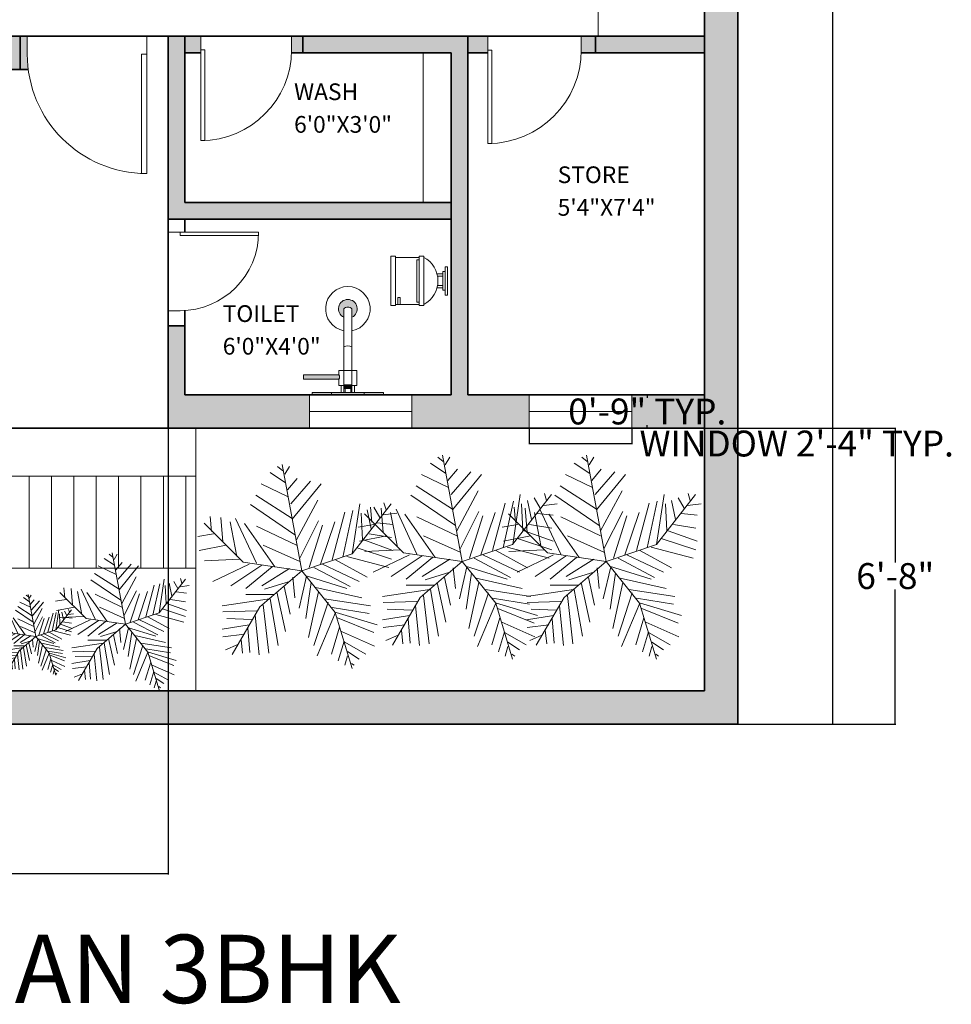
# Model space of a CAD drawing. Units: inches. Extents: x 1319 to 2030, y 219 to 1069.
# Tile 22 of 28: x 1776 to 2028, y 219 to 486. Entities that reach past the tile are written whole.
import ezdxf

# ---------------------------------------------------------------- set-up
doc = ezdxf.new("R2010")
doc.units = ezdxf.units.IN
doc.header["$MEASUREMENT"] = 0
doc.layers.get('0').update_dxf_attribs({"color": 12})
for name, color, linetype, lineweight in [('A-ANNO-DIMS', 2, 'Continuous', 18), ('A-AREA-IDEN', 250, 'Continuous', 18), ('A-FLOR', 8, 'Continuous', 18), ('A-FLOR-CASE', 8, 'Continuous', 18), ('A-FLOR-PATT', 41, 'Continuous', 13), ('A-GLAZ', 4, 'Continuous', 18), ('A-WALL-PATT', 252, 'Continuous', 13), ('C-PROP', 7, 'Continuous', 35), ('doors', 252, 'Continuous', 18), ('lawn', 82, 'Continuous', 13), ('PLUMBING FIXTURES', 252, 'Continuous', 18), ('text', 7, 'Continuous', 25), ('walls', 250, 'Continuous', 35)]:
    doc.layers.add(name, color=color, linetype=linetype, lineweight=lineweight)
doc.styles.get("Standard").update_dxf_attribs({"font": 'arial.ttf'})
doc.dimstyles.get("Standard").update_dxf_attribs({"dimtxt": 7, "dimasz": 0.18, "dimexe": 0.18, "dimexo": 0.0625, "dimgap": 0.09, "dimtad": 0, "dimtih": 1, "dimtoh": 1, "dimzin": 0, "dimdsep": 46, "dimlunit": 3, "dimtxsty": 'Standard', "dimcen": 0.09, "dimadec": 0, "dimazin": 0, "dimtfac": 1, "dimtofl": 0, "dimtmove": 0, "dimatfit": 3, "dimfxl": 1, "dimtolj": 1, "dimtzin": 0, "dimarcsym": 0})

# ---------------------------------------------------------------- blocks, each defined once
blk = doc.blocks.new('*U2')
for p, q in [((0, 0), (0, -6)), ((40, 0), (40, -6))]:
    blk.add_line(p, q)
blk.add_lwpolyline([(0, 0), (0, 40), (1.75, 40), (1.75, 0)], close=True)
blk.add_arc((0, 0), 40, 0, 90)
blk = doc.blocks.new('O.H SHOWER-PL')
at = {"layer": 'PLUMBING FIXTURES'}
for points in [[(-1.84, 0), (-1.84, -0.25), (1.84, -0.25), (1.84, 0)], [(0.46, -8.72), (0.46, -9.67, -0.422337), (-0.46, -9.67), (-0.46, -8.72, 4.325472)]]:
    blk.add_hatch(color=256, dxfattribs=at).paths.add_polyline_path(points)
for p, q in [((-1.84, 0), (-1.84, -0.25)), ((1.84, 0), (-1.84, 0)), ((1.84, 0), (1.84, -0.25)), ((1.84, -0.25), (-1.84, -0.25)), ((-0.46, -0.25), (-0.46, -9.67)), ((0.46, -0.25), (0.46, -9.67))]:
    blk.add_line(p, q, dxfattribs=at)
for centre, radius, start, end in [((0, -4.48), 1.03, 243.53, 296.47), ((0, -9.67), 2.5, 100.61, 79.39), ((0, -9.67), 1.05, 116.0349, 63.9652), ((0, -9.22), 0.643, 224.2078, 315.7922)]:
    blk.add_arc(centre, radius, start, end, dxfattribs=at)
blk = doc.blocks.new('DIVERTER-PL')
at = {"layer": 'PLUMBING FIXTURES'}
for points in [[(4, 0), (-4, 0), (-4, -0.25), (4, -0.25)], [(0.38, -1.14), (0.38, -0.7), (-0.37, -0.7), (-0.37, -1.14)], [(1, -1.75, 0.30818), (1, -2.25), (5, -2.25), (5, -1.75)]]:
    blk.add_hatch(color=256, dxfattribs=at).paths.add_polyline_path(points)
for p, q in [((-4, 0), (-4, -0.25)), ((-4, 0), (4, 0)), ((4, 0), (4, -0.25)), ((-4, -0.25), (4, -0.25)), ((-4, -0.25), (4, -0.25)), ((-1, -1.05), (-0.37, -1.05)), ((-1, -1.05), (-1, -2.75)), ((-0.75, -0.25), (-0.75, -1.05)), ((-0.37, -0.7), (0.38, -0.7)), ((-0.37, -0.7), (-0.37, -1.14)), ((-0.32, -0.7), (-0.32, -0.25)), ((0.32, -0.7), (0.32, -0.25)), ((0.38, -0.7), (0.38, -1.14)), ((0.38, -1.05), (1, -1.05)), ((0.75, -0.25), (0.75, -1.05)), ((1, -1.05), (1, -1.75)), ((-0.37, -1.14), (0.38, -1.14)), ((-1, -2.75), (1, -2.75)), ((1, -2.25), (1, -2.75))]:
    blk.add_line(p, q, dxfattribs=at)
at = {"layer": 'PLUMBING FIXTURES', "ltscale": 12}
for p, q in [((1, -1.75), (5, -1.75)), ((5, -2.25), (5, -1.75)), ((1, -2.25), (5, -2.25))]:
    blk.add_line(p, q, dxfattribs=at)
at = {"layer": 'PLUMBING FIXTURES'}
blk.add_arc((1.37, -2), 0.444, 145.7435, 214.2565, dxfattribs=at)
blk = doc.blocks.new('A$C7F153053')
at = {"layer": 'PLUMBING FIXTURES', "xscale": -1, "rotation": 270}
for name in ['DIVERTER-PL', 'O.H SHOWER-PL']:
    blk.add_blockref(name, (12.17, 4), dxfattribs=at)
blk = doc.blocks.new('*U25')
for p, q in [((-10, 22), (-10, 12)), ((-10, 21), (-7, 21)), ((-7, 21), (-7, 20)), ((10, 12), (10, 22)), ((-7, 20), (-10, 20)), ((9, 13), (-9, 13)), ((-9, 13), (-9, 12)), ((9, 12), (9, 13)), ((10.5, 12), (-10.5, 12)), ((-10.5, 10), (-10.5, 12)), ((10.5, 10), (-10.5, 10)), ((10.5, 12), (10.5, 10)), ((-3, 4.4065), (-3, 2)), ((3, 2), (3, 4.4065)), ((4, 2), (-4, 2)), ((-4, 2), (-4, 1)), ((-2, 2), (-2, 4.1658)), ((2, 4.1658), (2, 2)), ((4, 1), (4, 2))]:
    blk.add_line(p, q)
for points in [[(10.5, 22), (10.5, 24), (-10.5, 24), (-10.5, 22)], [(6, 0), (6, 1), (-6, 1), (-6, 0)]]:
    blk.add_lwpolyline(points, close=True)
blk.add_arc((0, 15.3333), 11.3333, 208.0725, 331.9275)
blk = doc.blocks.new('*U27')
for p, q in [((-10.186, 53.64), (-13.084, 55.962)), ((0, 0), (-10.5, 57)), ((-9.099, 51.782), (-6.563, 55.962)), ((-8.737, 47.138), (-17.069, 52.711)), ((-7.65, 43.423), (-2.578, 49.46)), ((-5.839, 35.992), (4.667, 48.067)), ((-7.288, 39.707), (-21.778, 46.673)), ((-5.114, 27.632), (10.463, 46.673)), ((-5.114, 28.097), (-24.676, 40.636)), ((-2.941, 16.486), (8.652, 37.85)), ((-3.665, 19.273), (-27.574, 35.527)), ((22.055, 7.198), (27.489, 32.277)), ((27, 9), (48, 36)), ((27.127, 9.056), (31.112, 35.992)), ((35.096, 32.741), (37.27, 22.524)), ((38.719, 34.134), (41.979, 28.561)), ((44.153, 36.456), (45.239, 32.741)), ((-48.585, 21.131), (-49.309, 29.026)), ((-43.513, 28.561), (-42.427, 15.558)), ((-35.544, 28.097), (-24.314, 3.947)), ((-1.129, 6.734), (9.014, 26.704)), ((16.259, 5.805), (23.142, 31.348)), ((31.836, 30.883), (32.561, 16.486)), ((43.791, 29.954), (51.036, 30.883)), ((-31.5, 4.5), (-52.5, 25.5)), ((-38.442, 26.239), (-34.819, 7.663)), ((-14.533, 2.09), (-30.834, 25.31)), ((-24.314, 23.917), (-2.941, 13.7)), ((3.942, 1.625), (11.187, 24.381)), ((10.101, 3.483), (17.708, 26.239)), ((40.53, 25.775), (48.862, 24.846)), ((-47.498, 19.737), (-55.83, 18.344)), ((33.285, 16.486), (48.862, 10.913)), ((36.183, 19.737), (48.137, 17.88)), ((-40.615, 13.7), (-55.105, 10.913)), ((-20.691, 13.7), (-1.129, 4.876)), ((29.662, 12.307), (48.137, 6.269)), ((-33.37, 6.269), (-52.207, 5.34)), ((0, 0), (27, 9)), ((18.07, 5.805), (35.096, -3.483)), ((24.229, 7.663), (46.688, 1.625)), ((-28.299, 3.483), (-47.86, -5.805)), ((-21.416, 3.018), (-38.079, -8.128)), ((0, 0), (-31.5, 4.5)), ((-15.982, 2.09), (-30.11, -9.521)), ((0, 0), (-22.5, -19.5)), ((-6.563, 1.161), (-21.416, -8.128)), ((0, 0), (18, -22.5)), ((6.478, 1.625), (26.04, -8.592)), ((11.187, 3.483), (30.749, -5.805)), ((-4.752, -3.483), (-3.665, -14.629)), ((2.493, -3.019), (-1.491, -20.202)), ((1.769, -2.555), (24.229, -9.521)), ((-6.563, -5.805), (-19.967, -9.985)), ((-9.461, -8.592), (-6.201, -23.453)), ((5.029, -6.27), (2.131, -25.775)), ((7.565, -9.056), (32.198, -14.629)), ((-17.431, -15.094), (-42.789, -18.809)), ((-15.257, -12.772), (-30.11, -12.772)), ((-17.069, -15.094), (-12.721, -40.172)), ((-13.446, -11.378), (-8.737, -32.741)), ((9.014, -11.378), (3.58, -35.992)), ((12.274, -15.094), (36.907, -18.809)), ((-22.5, -19.5), (-37.5, -45)), ((-20.691, -18.345), (-17.793, -44.352)), ((14.085, -16.951), (6.478, -40.172)), ((16.259, -19.738), (36.183, -22.989)), ((-24.314, -21.596), (-42.427, -22.06)), ((-26.849, -26.24), (-40.253, -25.775)), ((-25.038, -23.918), (-22.865, -45.281)), ((18.07, -22.524), (8.289, -45.745)), ((18, -22.5), (27, -52.5)), ((18.433, -22.524), (40.53, -29.026)), ((19.157, -25.311), (38.719, -33.206)), ((-28.299, -29.026), (-42.789, -31.348)), ((-29.023, -30.884), (-27.936, -43.887)), ((20.244, -30.419), (15.897, -44.816)), ((-30.834, -34.135), (-42.427, -35.528)), ((-32.646, -36.921), (-31.921, -44.352)), ((21.331, -32.741), (39.081, -40.636)), ((-34.457, -39.708), (-40.978, -42.494)), ((22.78, -37.85), (19.519, -48.532)), ((22.78, -38.314), (34.372, -44.816)), ((24.591, -45.745), (23.142, -50.854)), ((24.591, -43.423), (30.749, -47.603)), ((26.764, -49.925), (28.213, -50.854))]:
    blk.add_line(p, q)
blk = doc.blocks.new('*D29')
at = {"layer": 'A-ANNO-DIMS', "color": 0, "lineweight": -2, "transparency": 16777216}
for p, q in [((1995.58, 955.23), (1995.33, 955.23)), ((1995.51, 955.05), (1995.51, 628.88)), ((1995.51, 295.41), (1995.51, 621.58)), ((1995.58, 295.23), (1995.33, 295.23))]:
    blk.add_line(p, q, dxfattribs=at)
at = {"layer": 'A-ANNO-DIMS', "color": 0, "transparency": 16777216}
for points in [[(1995.48, 955.05), (1995.54, 955.05), (1995.51, 955.23)], [(1995.48, 295.41), (1995.54, 295.41), (1995.51, 295.23)]]:
    blk.add_solid(points, dxfattribs=at)
at = {"layer": 'Defpoints', "color": 0, "transparency": 16777216}
for p in [(1995.64, 955.23), (1995.51, 295.23), (1995.64, 295.23)]:
    blk.add_point(p, dxfattribs=at)
at = {"layer": 'A-ANNO-DIMS', "color": 0, "transparency": 16777216, "insert": (1995.51, 625.23), "char_height": 7, "attachment_point": 5}
blk.add_mtext("\\A1;55'", dxfattribs=at)
blk = doc.blocks.new('WIN-28')
for p, q in [((0, 9), (0, 0)), ((27.75, 9), (0, 9)), ((0, 9), (0, 4.5)), ((27.75, 0), (27.75, 9)), ((0, 4.5), (27.75, 4.5)), ((0, 0), (27.75, 0))]:
    blk.add_line(p, q)
blk = doc.blocks.new('*D52')
at = {"layer": 'A-ANNO-DIMS', "color": 0, "lineweight": -2, "transparency": 16777216}
for p, q in [((1913.44, 375.16), (1913.44, 370.88)), ((1941.19, 375.16), (1941.19, 370.88)), ((1913.62, 371.06), (1941.01, 371.06)), ((1941.19, 371.06), (1941.37, 371.06))]:
    blk.add_line(p, q, dxfattribs=at)
at = {"layer": 'A-ANNO-DIMS', "color": 0, "transparency": 16777216}
for points in [[(1913.62, 371.09), (1913.62, 371.03), (1913.44, 371.06)], [(1941.01, 371.09), (1941.01, 371.03), (1941.19, 371.06)]]:
    blk.add_solid(points, dxfattribs=at)
at = {"layer": 'Defpoints', "color": 0, "transparency": 16777216}
for p in [(1913.44, 375.23), (1941.19, 375.23), (1941.19, 371.06)]:
    blk.add_point(p, dxfattribs=at)
at = {"layer": 'A-ANNO-DIMS', "color": 0, "transparency": 16777216, "insert": (1985.75, 371.06), "char_height": 7, "attachment_point": 5}
blk.add_mtext('\\A1;WINDOW 2\'-4" TYP.', dxfattribs=at)
blk = doc.blocks.new('*D53')
at = {"layer": 'A-ANNO-DIMS', "color": 0, "lineweight": -2, "transparency": 16777216}
for p, q in [((1941.25, 384.23), (1945.53, 384.23)), ((1945.35, 384.05), (1945.35, 383.39)), ((1945.35, 375.41), (1945.35, 376.06)), ((1941.25, 375.23), (1945.53, 375.23))]:
    blk.add_line(p, q, dxfattribs=at)
at = {"layer": 'A-ANNO-DIMS', "color": 0, "transparency": 16777216}
for points in [[(1945.32, 384.05), (1945.38, 384.05), (1945.35, 384.23)], [(1945.32, 375.41), (1945.38, 375.41), (1945.35, 375.23)]]:
    blk.add_solid(points, dxfattribs=at)
at = {"layer": 'Defpoints', "color": 0, "transparency": 16777216}
for p in [(1941.19, 384.23), (1945.35, 384.23), (1941.19, 375.23)]:
    blk.add_point(p, dxfattribs=at)
at = {"layer": 'A-ANNO-DIMS', "color": 0, "transparency": 16777216, "insert": (1945.35, 379.73), "char_height": 7, "attachment_point": 5}
blk.add_mtext('\\A1;0\'-9" TYP.', dxfattribs=at)
blk = doc.blocks.new('*D64')
at = {"layer": 'A-ANNO-DIMS', "color": 0, "lineweight": -2, "transparency": 16777216}
for p, q in [((1648.34, 375.16), (1648.34, 254.5)), ((1815.84, 375.16), (1815.84, 254.5)), ((1648.52, 254.68), (1709.43, 254.68)), ((1815.66, 254.68), (1754.75, 254.68))]:
    blk.add_line(p, q, dxfattribs=at)
at = {"layer": 'A-ANNO-DIMS', "color": 0, "transparency": 16777216}
for points in [[(1648.52, 254.71), (1648.52, 254.65), (1648.34, 254.68)], [(1815.66, 254.71), (1815.66, 254.65), (1815.84, 254.68)]]:
    blk.add_solid(points, dxfattribs=at)
at = {"layer": 'Defpoints', "color": 0, "transparency": 16777216}
for p in [(1648.34, 375.23), (1815.84, 375.23), (1815.84, 254.68)]:
    blk.add_point(p, dxfattribs=at)
at = {"layer": 'A-ANNO-DIMS', "color": 0, "transparency": 16777216, "insert": (1732.09, 254.68), "char_height": 7, "attachment_point": 5}
blk.add_mtext('\\A1;13\'-11 1/2"', dxfattribs=at)
blk = doc.blocks.new('*D66')
at = {"layer": 'A-ANNO-DIMS', "color": 0, "lineweight": -2, "transparency": 16777216}
for p, q in [((1960.91, 375.23), (2012.57, 375.23)), ((2012.39, 375.05), (2012.39, 338.89)), ((2012.39, 295.41), (2012.39, 331.56)), ((1969.91, 295.23), (2012.57, 295.23))]:
    blk.add_line(p, q, dxfattribs=at)
at = {"layer": 'A-ANNO-DIMS', "color": 0, "transparency": 16777216}
for points in [[(2012.36, 375.05), (2012.42, 375.05), (2012.39, 375.23)], [(2012.36, 295.41), (2012.42, 295.41), (2012.39, 295.23)]]:
    blk.add_solid(points, dxfattribs=at)
at = {"layer": 'Defpoints', "color": 0, "transparency": 16777216}
for p in [(1960.84, 375.23), (2012.39, 375.23), (1969.84, 295.23)]:
    blk.add_point(p, dxfattribs=at)
at = {"layer": 'A-ANNO-DIMS', "color": 0, "transparency": 16777216, "insert": (2012.39, 335.23), "char_height": 7, "attachment_point": 5}
blk.add_mtext('\\A1;6\'-8"', dxfattribs=at)

msp = doc.modelspace()

# ---------------------------------------------------------------- hatches: boundary and pattern name
at = {"layer": 'A-FLOR-PATT'}
h = msp.add_hatch(dxfattribs=at)
h.set_pattern_fill('ANSI31', color=256, scale=48.3872, angle=45, style=0)
h.paths.add_polyline_path([(1578.343, 337.406), (1823.279, 337.406), (1823.279, 362.242), (1769.593, 362.242), (1769.593, 375.227), (1578.343, 375.227)])
at = {"layer": 'A-WALL-PATT'}
h = msp.add_hatch(color=256, dxfattribs=at)
h.dxf.hatch_style = 1
h.paths.add_polyline_path([(1378.843, 946.227), (1960.843, 946.227), (1960.843, 860.616), (1922.194, 860.616), (1922.194, 851.616), (1960.843, 851.616), (1960.843, 304.227), (1578.343, 304.227), (1578.343, 295.227), (1969.843, 295.227), (1969.843, 955.227), (1369.843, 955.227), (1369.843, 295.227), (1378.843, 295.227)])
h = msp.add_hatch(color=256, dxfattribs=at)
h.dxf.hatch_style = 1
h.paths.add_polyline_path([(1856.292, 860.616), (1812.343, 860.616), (1812.343, 851.616), (1812.343, 700.993), (1816.843, 700.993), (1816.843, 851.616), (1856.292, 851.616)])
h.paths.add_polyline_path([(1960.843, 663.616), (1812.343, 663.616), (1782.783, 663.616), (1782.783, 659.116), (1812.343, 659.116), (1960.843, 659.116)])
h.paths.add_polyline_path([(1857.424, 659.116), (1852.924, 659.116), (1852.924, 616.807), (1857.424, 616.807)])
h.paths.add_polyline_path([(1735.843, 661.727), (1731.843, 661.727), (1636.133, 661.727), (1636.133, 657.227), (1731.343, 657.227), (1731.343, 481.227), (1618.616, 481.227), (1618.616, 472.227), (1639.343, 472.227), (1639.343, 384.227), (1627.044, 384.227), (1627.044, 375.227), (1648.343, 375.227), (1648.343, 384.227), (1648.343, 472.227), (1750.706, 472.227), (1750.706, 481.227), (1735.843, 481.227), (1735.843, 657.727)])
h.paths.add_polyline_path([(1587.343, 481.227), (1578.343, 481.227), (1578.343, 375.227), (1597.622, 375.227), (1597.622, 384.227), (1587.343, 384.227)])
h.paths.add_polyline_path([(1769.593, 384.227), (1693.482, 384.227), (1693.482, 375.227), (1769.593, 375.227)])
h.paths.add_polyline_path([(1775.828, 481.227), (1765.831, 481.227), (1765.831, 472.227), (1775.828, 472.227)])
h.paths.add_polyline_path([(1824.625, 481.227), (1820.343, 481.227), (1820.343, 476.727), (1824.625, 476.727), (1824.625, 477.545)], flags=0)
h.paths.add_polyline_path([(1896.843, 481.227), (1852.26, 481.227), (1852.26, 476.727), (1892.343, 476.727), (1892.343, 384.227), (1881.742, 384.227), (1881.742, 375.227), (1913.435, 375.227), (1913.435, 384.227), (1896.843, 384.227)])
h.paths.add_polyline_path([(1960.843, 481.227), (1931.341, 481.227), (1931.341, 476.727), (1960.843, 476.727)])
h.paths.add_polyline_path([(1736.343, 918.227), (1731.843, 918.227), (1731.843, 890.227), (1582.843, 890.227), (1582.843, 781.727), (1582.843, 769.171), (1587.343, 769.171), (1587.343, 781.727), (1587.343, 885.727), (1731.843, 885.727), (1731.843, 851.616), (1736.343, 851.616), (1736.343, 890.227)])
h.paths.add_polyline_path([(1781.022, 860.616), (1773.021, 860.616, -0.0322281), (1773.289, 856.464), (1773.289, 851.616), (1781.022, 851.616)])
h.paths.add_polyline_path([(1587.343, 946.227), (1582.843, 946.227), (1582.843, 926.136), (1587.343, 926.136)])
h.paths.add_polyline_path([(1647.843, 946.227), (1643.343, 946.227), (1643.343, 926.136), (1647.843, 926.136)])
h.paths.add_polyline_path([(1543.343, 786.227), (1429.843, 786.227), (1429.843, 757.555), (1434.343, 757.555), (1438.843, 757.555), (1438.843, 781.727), (1543.343, 781.727)])
h.paths.add_polyline_path([(1543.343, 781.727), (1538.843, 781.727), (1538.843, 709.727), (1534.597, 709.727), (1534.597, 705.227), (1543.343, 705.227), (1543.343, 709.727)])
h.paths.add_polyline_path([(1499.955, 709.727), (1438.843, 709.727), (1438.843, 734.463), (1429.843, 734.463), (1429.843, 552.227), (1470.241, 552.227), (1470.241, 561.227), (1438.843, 561.227), (1438.843, 705.227), (1499.955, 705.227)])
h.paths.add_polyline_path([(1587.343, 709.727), (1582.843, 709.727), (1582.843, 561.227), (1543.433, 561.227), (1543.433, 552.227), (1587.343, 552.227)])
h.paths.add_polyline_path([(1546.835, 709.727), (1543.343, 709.727), (1543.343, 705.227), (1546.835, 705.227)])
h.paths.add_polyline_path([(1582.843, 709.727), (1579.15, 709.727), (1579.15, 705.227), (1582.843, 705.227)], flags=17)
h.paths.add_polyline_path([(1548.368, 786.227), (1543.343, 786.227), (1543.343, 781.727), (1548.368, 781.727)])
h.paths.add_polyline_path([(1582.843, 786.227), (1580.683, 786.227), (1580.683, 781.727), (1582.843, 781.727)])
h.paths.add_polyline_path([(1587.343, 892.402), (1582.843, 892.402), (1582.843, 890.227), (1587.343, 890.227)], flags=17)
h.paths.add_polyline_path([(1647.843, 892.402), (1643.343, 892.402), (1643.343, 890.227), (1647.843, 890.227)], flags=17)
h.paths.add_polyline_path([(1740.974, 856.464), (1740.974, 860.616), (1736.343, 860.616), (1736.343, 851.616), (1740.974, 851.616)])
h.paths.add_polyline_path([(1853.989, 384.227), (1820.343, 384.227), (1820.343, 402.924), (1815.843, 402.924), (1815.843, 375.227), (1853.989, 375.227)])
h.paths.add_polyline_path([(1892.343, 436.227), (1820.343, 436.227), (1820.343, 481.227), (1815.843, 481.227), (1815.843, 431.727), (1892.343, 431.727)])
h.paths.add_polyline_path([(1849.175, 481.227), (1824.625, 481.227), (1824.625, 477.545), (1825.699, 477.545), (1825.699, 453.018, 0.4014527), (1849.175, 477.545)], flags=0)
h.paths.add_polyline_path([(1960.843, 384.227), (1941.188, 384.227), (1941.188, 375.227), (1960.843, 375.227)])
h.paths.add_polyline_path([(1902.267, 481.227), (1896.843, 481.227), (1896.843, 476.727), (1902.267, 476.727), (1902.267, 477.44)], flags=0)
h = msp.add_hatch(color=256, dxfattribs=at)
h.dxf.hatch_style = 1
h.paths.add_polyline_path([(1777.721, 476.38), (1777.721, 481.227), (1775.828, 481.227), (1775.828, 472.227), (1777.989, 472.227, -0.0322281)])
h.paths.add_polyline_path([(1852.26, 481.227), (1849.175, 481.227), (1849.175, 477.545, -0.008326), (1849.162, 476.727), (1852.26, 476.727)])
h.paths.add_polyline_path([(1902.267, 481.227), (1896.843, 481.227), (1896.843, 476.727), (1902.267, 476.727), (1902.267, 477.44)])
h.paths.add_polyline_path([(1931.341, 481.227), (1927.512, 481.227), (1927.512, 477.44, -0.007064), (1927.502, 476.727), (1931.341, 476.727)])
h = msp.add_hatch(color=256, dxfattribs=at)
h.dxf.hatch_style = 1
h.paths.add_polyline_path([(1824.625, 477.545), (1824.625, 481.227), (1820.343, 481.227), (1820.343, 476.727), (1824.625, 476.727)])

# ---------------------------------------------------------------- linework, layer by layer
at = {"layer": 'A-FLOR'}
for p, q in [((1823.279, 375.227), (1823.279, 304.227)), ((1769.593, 362.242), (1823.279, 362.242)), ((1394.092, 337.406), (1817.431, 337.406)), ((1823.279, 337.406), (1817.431, 337.406))]:
    msp.add_line(p, q, dxfattribs=at)
at = {"layer": 'A-FLOR-CASE'}
for p, q in [((1932.091, 631.139), (1932.091, 481.227)), ((1884.747, 476.727), (1884.747, 436.227))]:
    msp.add_line(p, q, dxfattribs=at)
at = {"layer": 'C-PROP'}
for p, q in [((1969.843, 955.227), (1969.843, 295.227)), ((1969.843, 295.227), (1369.843, 295.227))]:
    msp.add_line(p, q, dxfattribs=at)
at = {"layer": 'walls'}
for p, q in [((1960.843, 851.616), (1960.843, 304.227)), ((1735.843, 481.227), (1960.843, 481.227)), ((1775.828, 472.227), (1775.828, 481.227)), ((1815.843, 481.227), (1815.843, 375.227)), ((1820.343, 481.227), (1820.343, 436.227)), ((1852.26, 481.227), (1852.26, 476.727)), ((1896.843, 481.227), (1896.843, 384.227)), ((1931.341, 481.227), (1931.341, 476.727)), ((1820.343, 476.727), (1824.625, 476.727)), ((1849.162, 476.727), (1892.343, 476.727)), ((1892.343, 476.727), (1892.343, 384.227)), ((1896.843, 476.727), (1902.267, 476.727)), ((1927.502, 476.727), (1960.843, 476.727)), ((1648.343, 472.227), (1777.989, 472.227)), ((1820.343, 436.227), (1892.343, 436.227)), ((1815.843, 431.727), (1892.343, 431.727)), ((1820.343, 431.727), (1820.343, 428.227)), ((1820.343, 407.026), (1820.343, 384.227)), ((1815.843, 402.924), (1820.343, 402.924)), ((1820.343, 384.227), (1892.343, 384.227)), ((1896.843, 384.227), (1960.843, 384.227)), ((1578.343, 375.227), (1960.843, 375.227)), ((1960.843, 304.227), (1578.343, 304.227))]:
    msp.add_line(p, q, dxfattribs=at)

# ---------------------------------------------------------------- block references
at = {"layer": 'A-GLAZ'}
for p in [(1853.989, 375.227), (1913.435, 375.227)]:
    msp.add_blockref('WIN-28', p, dxfattribs=at)
at = {"layer": 'doors'}
for p, xscale, yscale, zscale, rotation in [((1810.036, 476.38), 0.8078659498341503, 0.8078659498341503, 0.8078659498341503, 180), ((1824.625, 477.545), -0.6137583830774199, 0.6137583830774199, 0.6137583830774199, 180), ((1902.267, 477.44), -0.6311292477256859, 0.6311292477256859, 0.6311292477256859, 180), ((1819.029, 428.227), 0.5310368015679418, 0.5310368015679418, 0.5310368015679418, 270)]:
    msp.add_blockref('*U2', p, dxfattribs=dict(at, xscale=xscale, yscale=yscale, zscale=zscale, rotation=rotation))
at = {"layer": 'lawn'}
for p, xscale, yscale, zscale in [((1895.308, 339.208), 0.5032398725192154, 0.5032398725192154, 0.5032398725192154), ((1934.219, 339.208), 0.5032398725192154, 0.5032398725192154, 0.5032398725192154), ((1851.952, 336.688), 0.5032398725192154, 0.5032398725192154, 0.5032398725192154), ((1804.26, 322.218), 0.3377350603606453, 0.3377350603606453, 0.3377350603606453), ((1780.073, 318.897), 0.1996319451716265, 0.1996319451716265, 0.1996319451716265)]:
    msp.add_blockref('*U27', p, dxfattribs=dict(at, xscale=xscale, yscale=yscale, zscale=zscale))
at = {"layer": 'PLUMBING FIXTURES', "rotation": 90}
for name, p, xscale, yscale, zscale in [('*U25', (1891.309, 415.039), 0.6365860877769962, 0.6365860877769962, 0.6365860877769962), ('A$C7F153053', (1874.026, 413.501), -2.406230429091579, 2.406230429091579, 2.406230429091579)]:
    msp.add_blockref(name, p, dxfattribs=dict(at, xscale=xscale, yscale=yscale, zscale=zscale))

# ---------------------------------------------------------------- texts
at = {"layer": 'A-AREA-IDEN'}
for s, p in [('WASH', (1849.87, 463.921)), ('6\'0"X3\'0"', (1849.87, 455.097)), ('STORE', (1921.126, 441.48)), ('5\'4"X7\'4"', (1921.126, 432.656)), ('TOILET', (1830.577, 403.936)), ('6\'0"X4\'0"', (1830.577, 395.112))]:
    msp.add_text(s, height=4.5146, dxfattribs=at).set_placement(p)
at = {"layer": 'text'}
msp.add_text('50X55 SOUTH FACE HOUSE PLAN 3BHK', height=18.48405, dxfattribs=at).set_placement((1420.923, 219.766))

# ---------------------------------------------------------------- dimensions: what is measured, and where the dimension line sits
at = {"layer": 'A-ANNO-DIMS'}
for base, p1, p2, override, picture, middle in [((1995.506, 295.227), (1995.643, 955.227), (1995.643, 295.227), {"dimclrd": 0, "dimclre": 0, "dimclrt": 0}, '*D29', (1995.506, 625.227)), ((2012.394, 375.227), (1969.843, 295.227), (1960.843, 375.227), {"dimdec": 1, "dimlfac": 1, "dimrnd": 0, "dimzin": 1, "dimdsep": 46, "dimlunit": 4, "dimfrac": 2}, '*D66', (2012.394, 335.227))]:
    dim = msp.add_linear_dim(base=base, p1=p1, p2=p2, angle=90, dimstyle='Standard', override=override, dxfattribs=at)
    dim.commit()
    dim.dimension.update_dxf_attribs({"geometry": picture, "text_midpoint": middle})
dim = msp.add_linear_dim(base=(1945.351, 384.227), p1=(1941.188, 375.227), p2=(1941.188, 384.227), angle=90, text='<> TYP.', dimstyle='Standard', override={"dimdec": 1, "dimlfac": 1, "dimrnd": 0, "dimzin": 1, "dimdsep": 46, "dimlunit": 4, "dimfrac": 2}, dxfattribs=at)
dim.commit()
dim.dimension.update_dxf_attribs({"geometry": '*D53', "text_midpoint": (1945.351, 379.727)})
dim = msp.add_linear_dim(base=(1941.188, 371.064), p1=(1913.435, 375.227), p2=(1941.188, 375.227), text='WINDOW <> TYP.', dimstyle='Standard', override={"dimdec": 1, "dimlfac": 1, "dimrnd": 0, "dimzin": 1, "dimdsep": 46, "dimlunit": 4, "dimfrac": 2}, dxfattribs=at)
dim.commit()
dim.dimension.update_dxf_attribs({"geometry": '*D52', "text_midpoint": (1985.748, 371.064)})
dim = msp.add_linear_dim(base=(1815.843, 254.677), p1=(1648.343, 375.227), p2=(1815.843, 375.227), dimstyle='Standard', override={"dimdec": 1, "dimlfac": 1, "dimrnd": 0, "dimzin": 1, "dimdsep": 46, "dimlunit": 4, "dimfrac": 2}, dxfattribs=at)
dim.commit()
dim.dimension.update_dxf_attribs({"geometry": '*D64', "text_midpoint": (1732.093, 254.677)})

doc.saveas('drawing.dxf')
